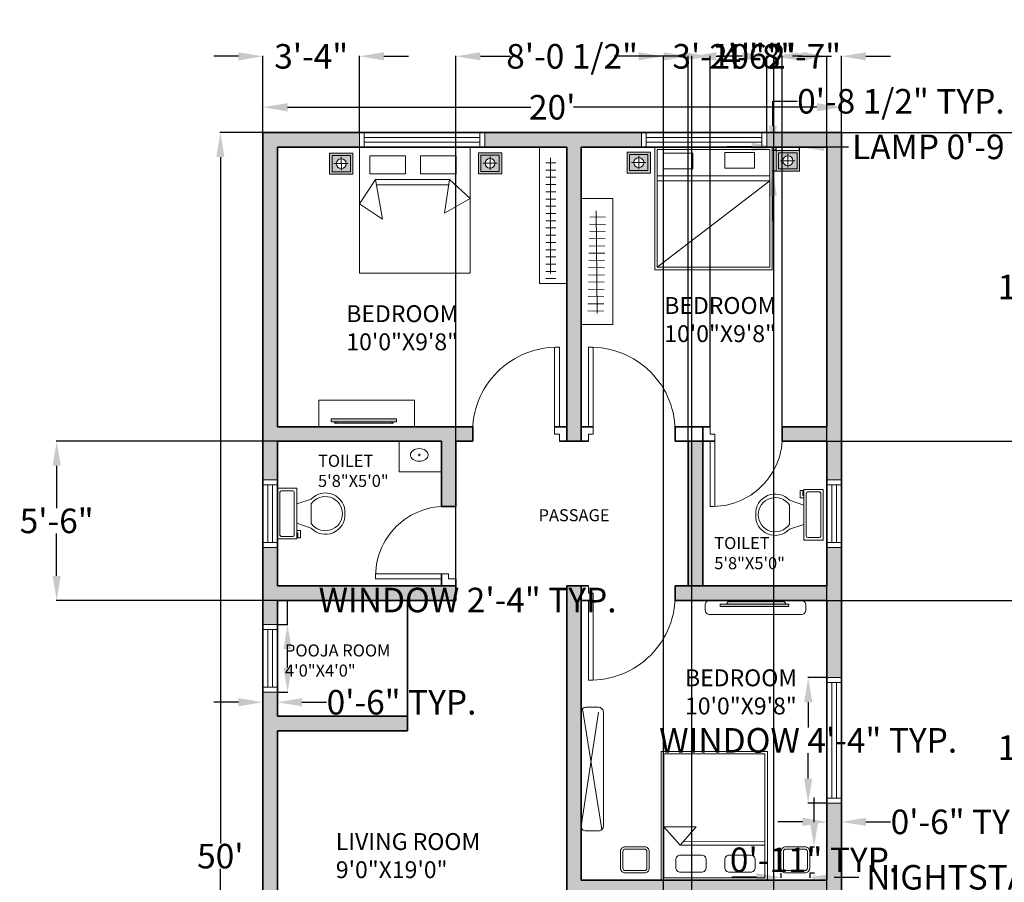
# Model space of a CAD drawing. Units: inches. Extents: x 1294 to 2470, y 659 to 1389.
# Tile 3 of 4: x 1306 to 1714, y 1031 to 1389. Entities that reach past the tile are written whole.
import ezdxf

# ---------------------------------------------------------------- set-up
doc = ezdxf.new("R2010")
doc.units = ezdxf.units.IN
doc.header["$MEASUREMENT"] = 0
for name, color, linetype, lineweight in [('A-ANNO-DIMS', 2, 'Continuous', 18), ('A-AREA-IDEN', 7, 'Continuous', 20), ('A-DOOR', 3, 'Continuous', 18), ('A-FLOR-CASE', 9, 'Continuous', 20), ('A-FLOR-FIXT', 9, 'Continuous', 18), ('A-FURN', 8, 'Continuous', 18), ('A-FURN-PATT', 9, 'Continuous', 13), ('A-GLAZ', 4, 'Continuous', 18), ('A-WALL', 7, 'Continuous', 35), ('A-WALL-PATT', 252, 'Continuous', 13)]:
    doc.layers.add(name, color=color, linetype=linetype, lineweight=lineweight)
doc.styles.get("Standard").update_dxf_attribs({"font": 'arial.ttf'})
doc.dimstyles.get("Standard").update_dxf_attribs({"dimtxt": 10.18, "dimasz": 10.18, "dimexe": 0.18, "dimexo": 0.0625, "dimgap": 0.09, "dimtad": 0, "dimtih": 1, "dimtoh": 1, "dimdec": 0, "dimzin": 0, "dimdsep": 46, "dimlunit": 3, "dimtxsty": 'Standard', "dimcen": 0.09, "dimadec": 0, "dimazin": 0, "dimtfac": 1, "dimtdec": 0, "dimtofl": 0, "dimtmove": 0, "dimatfit": 3, "dimfxl": 1, "dimtolj": 1, "dimtzin": 0, "dimarcsym": 0})

# ---------------------------------------------------------------- blocks, each defined once
blk = doc.blocks.new('*U2')
for p, q in [((9.5, -6), (9.5, -2)), ((-8, -8.5), (-8, -8)), ((-7, -8), (-7, -9.5)), ((-4, -8), (-6, -14)), ((4, -8), (6, -14)), ((-10, -8.5), (-8, -8.5)), ((-10, -9.5), (-10, -8.5)), ((-7, -9.5), (-10, -9.5)), ((4, -14), (-4, -14))]:
    blk.add_line(p, q)
blk.add_lwpolyline([(10.5, -8), (10.5, 0), (-10.5, 0), (-10.5, -8)], close=True)
for points in [[(-9.5, -2), (-9.5, -6)], [(8.5, -1), (-8.5, -1)], [(-8.5, -7), (8.5, -7)]]:
    blk.add_lwpolyline(points)
for centre, radius, start, end in [((-8.625, -1.875), 0.8839, 81.8699, 188.1301), ((8.625, -1.875), 0.8839, 351.8699, 98.1301), ((-8.625, -6.125), 0.8839, 171.869898, 278.1301), ((8.625, -6.125), 0.8839, 261.8699, 8.1301), ((-0.4772, -19.9188), 8.0953, 133.01722, 273.38), ((0.0374, -19.8731), 7.127, 124.50543, 269.7), ((-0.0373, -19.8731), 7.127, 270.3, 55.4946), ((0.4773, -19.9188), 8.0953, 266.62, 46.9828)]:
    blk.add_arc(centre, radius, start, end)
blk = doc.blocks.new('*D6')
at = {"layer": 'A-ANNO-DIMS', "color": 0, "lineweight": -2, "transparency": 16777216}
for p, q in [((1406.6, 1341.78), (1388.79, 1341.78)), ((1388.97, 1331.6), (1388.97, 1047.07)), ((1388.97, 751.96), (1388.97, 1036.5)), ((1406.6, 741.78), (1388.79, 741.78))]:
    blk.add_line(p, q, dxfattribs=at)
at = {"layer": 'A-ANNO-DIMS', "color": 0, "transparency": 16777216}
for points in [[(1387.28, 1331.6), (1390.67, 1331.6), (1388.97, 1341.78)], [(1387.28, 751.96), (1390.67, 751.96), (1388.97, 741.78)]]:
    blk.add_solid(points, dxfattribs=at)
at = {"layer": 'Defpoints', "color": 0, "transparency": 16777216}
for p in [(1406.66, 1341.78), (1388.97, 741.78), (1406.66, 741.78)]:
    blk.add_point(p, dxfattribs=at)
at = {"layer": 'A-ANNO-DIMS', "color": 0, "transparency": 16777216, "insert": (1388.97, 1041.78), "char_height": 10.18, "attachment_point": 5}
blk.add_mtext("\\A1;50'", dxfattribs=at)
blk = doc.blocks.new('*D7')
at = {"layer": 'A-ANNO-DIMS', "color": 0, "lineweight": -2, "transparency": 16777216}
for p, q in [((1406.66, 1341.85), (1406.66, 1352.45)), ((1416.84, 1352.27), (1517.85, 1352.27)), ((1636.48, 1352.27), (1535.48, 1352.27)), ((1646.66, 1341.85), (1646.66, 1352.45))]:
    blk.add_line(p, q, dxfattribs=at)
at = {"layer": 'A-ANNO-DIMS', "color": 0, "transparency": 16777216}
for points in [[(1416.84, 1353.97), (1416.84, 1350.57), (1406.66, 1352.27)], [(1636.48, 1353.97), (1636.48, 1350.57), (1646.66, 1352.27)]]:
    blk.add_solid(points, dxfattribs=at)
at = {"layer": 'Defpoints', "color": 0, "transparency": 16777216}
for p in [(1646.66, 1352.27), (1406.66, 1341.78), (1646.66, 1341.78)]:
    blk.add_point(p, dxfattribs=at)
at = {"layer": 'A-ANNO-DIMS', "color": 0, "transparency": 16777216, "insert": (1526.66, 1352.27), "char_height": 10.18, "attachment_point": 5}
blk.add_mtext("\\A1;20'", dxfattribs=at)
blk = doc.blocks.new('DOOR-SWING-36')
for p, q in [((34.01, 0), (34.01, 36)), ((36.01, 3), (36.01, 36)), ((34.01, 0), (36.01, 0))]:
    blk.add_line(p, q)
blk.add_arc((35.01, 1), 35.01, 88.3634, 181.6366)
blk = doc.blocks.new('WIN-48')
for p, q in [((0, 6), (0, 0)), ((2, 6), (2, 0)), ((50, 6), (50, 0)), ((52, 6), (52, 0)), ((50, 4), (2, 4)), ((50, 2), (2, 2))]:
    blk.add_line(p, q)
blk = doc.blocks.new('WIN-24')
for p, q in [((6, 28), (0, 28)), ((6, 26), (0, 26)), ((2, 26), (2, 2)), ((4, 26), (4, 2)), ((6, 2), (0, 2)), ((6, 0), (0, 0))]:
    blk.add_line(p, q)
blk = doc.blocks.new('NIGHTSTAND-LAMP')
h = blk.add_hatch(color=256)
h.dxf.hatch_style = 1
h.paths.add_polyline_path([(1, 7.67), (1, 1), (8.65, 1), (8.65, 7.67)], flags=0)
h.paths.add_polyline_path([(6.89, 4.34, -1), (2.76, 4.34, -1)], flags=0)
h.paths.add_polyline_path([(0, 8.67), (0, 0), (9.65, 0), (9.65, 8.67)])
h.paths.add_polyline_path([(8.65, 7.67), (8.65, 1), (1, 1), (1, 7.67)], flags=16)
h = blk.add_hatch(color=256)
h.dxf.hatch_style = 1
h.paths.add_polyline_path([(1, 7.67), (1, 1), (8.65, 1), (8.65, 7.67)])
h.paths.add_polyline_path([(6.89, 4.34, -1), (2.76, 4.34, -1)], flags=16)
for p, q in [((1.82, 4.38), (7.72, 4.39)), ((4.83, 7.2), (4.87, 1.61))]:
    blk.add_line(p, q)
for points in [[(9.65, 8.67), (0, 8.67), (0, 0), (9.65, 0)], [(8.65, 7.67), (1, 7.67), (1, 1), (8.65, 1)]]:
    blk.add_lwpolyline(points, close=True)
blk.add_circle((4.83, 4.34), 2.06)
blk = doc.blocks.new('NIGHTSTAND-RECT')
for points in [[(0, 8.9, -0.414214), (2, 10.9), (9.94, 10.9, -0.414214), (11.94, 8.9), (11.94, 2, -0.414214), (9.94, 0), (2, 0, -0.414214), (0, 2)], [(1, 8.9, -0.414214), (2, 9.9), (9.94, 9.9, -0.414214), (10.94, 8.9), (10.94, 2, -0.414214), (9.94, 1), (2, 1, -0.414214), (1, 2)]]:
    blk.add_lwpolyline(points, format="xyb", close=True)
blk = doc.blocks.new('*D18')
at = {"layer": 'A-ANNO-DIMS', "color": 0, "lineweight": -2, "transparency": 16777216}
for p, q in [((1640.6, 1115.78), (1632.68, 1115.78)), ((1632.86, 1105.6), (1632.86, 1095.14)), ((1632.86, 1073.96), (1632.86, 1084.43)), ((1640.6, 1063.78), (1632.68, 1063.78))]:
    blk.add_line(p, q, dxfattribs=at)
at = {"layer": 'A-ANNO-DIMS', "color": 0, "transparency": 16777216}
for points in [[(1631.17, 1105.6), (1634.56, 1105.6), (1632.86, 1115.78)], [(1631.17, 1073.96), (1634.56, 1073.96), (1632.86, 1063.78)]]:
    blk.add_solid(points, dxfattribs=at)
at = {"layer": 'Defpoints', "color": 0, "transparency": 16777216}
for p in [(1640.66, 1115.78), (1632.86, 1063.78), (1640.66, 1063.78)]:
    blk.add_point(p, dxfattribs=at)
at = {"layer": 'A-ANNO-DIMS', "color": 0, "transparency": 16777216, "insert": (1632.86, 1089.78), "char_height": 10.18, "attachment_point": 5}
blk.add_mtext('\\A1;WINDOW 4\'-4" TYP.', dxfattribs=at)
blk = doc.blocks.new('*D19')
at = {"layer": 'A-ANNO-DIMS', "color": 0, "lineweight": -2, "transparency": 16777216}
for p, q in [((1640.66, 1063.72), (1640.66, 1055.8)), ((1646.66, 1063.72), (1646.66, 1055.8)), ((1630.48, 1055.98), (1620.3, 1055.98)), ((1656.84, 1055.98), (1667.02, 1055.98))]:
    blk.add_line(p, q, dxfattribs=at)
at = {"layer": 'A-ANNO-DIMS', "color": 0, "transparency": 16777216}
for points in [[(1630.48, 1057.68), (1630.48, 1054.29), (1640.66, 1055.98)], [(1656.84, 1057.68), (1656.84, 1054.29), (1646.66, 1055.98)]]:
    blk.add_solid(points, dxfattribs=at)
at = {"layer": 'Defpoints', "color": 0, "transparency": 16777216}
for p in [(1640.66, 1063.78), (1646.66, 1063.78), (1646.66, 1055.98)]:
    blk.add_point(p, dxfattribs=at)
at = {"layer": 'A-ANNO-DIMS', "color": 0, "transparency": 16777216, "insert": (1698.14, 1055.98), "char_height": 10.18, "attachment_point": 5}
blk.add_mtext('\\A1;0\'-6" TYP.', dxfattribs=at)
blk = doc.blocks.new('*D20')
at = {"layer": 'A-ANNO-DIMS', "color": 0, "lineweight": -2, "transparency": 16777216}
for p, q in [((1416.86, 1137.78), (1416.86, 1147.96)), ((1416.86, 1147.96), (1427.04, 1147.96)), ((1412.72, 1137.78), (1417.04, 1137.78)), ((1416.86, 1119.96), (1416.86, 1127.6)), ((1412.72, 1109.78), (1417.04, 1109.78))]:
    blk.add_line(p, q, dxfattribs=at)
at = {"layer": 'A-ANNO-DIMS', "color": 0, "transparency": 16777216}
for points in [[(1415.17, 1127.6), (1418.56, 1127.6), (1416.86, 1137.78)], [(1415.17, 1119.96), (1418.56, 1119.96), (1416.86, 1109.78)]]:
    blk.add_solid(points, dxfattribs=at)
at = {"layer": 'Defpoints', "color": 0, "transparency": 16777216}
for p in [(1412.66, 1137.78), (1416.86, 1137.78), (1412.66, 1109.78)]:
    blk.add_point(p, dxfattribs=at)
at = {"layer": 'A-ANNO-DIMS', "color": 0, "transparency": 16777216, "insert": (1491.54, 1147.96), "char_height": 10.18, "attachment_point": 5}
blk.add_mtext('\\A1;WINDOW 2\'-4" TYP.', dxfattribs=at)
blk = doc.blocks.new('*D21')
at = {"layer": 'A-ANNO-DIMS', "color": 0, "lineweight": -2, "transparency": 16777216}
for p, q in [((1406.66, 1109.72), (1406.66, 1105.4)), ((1412.66, 1109.72), (1412.66, 1105.4)), ((1396.48, 1105.58), (1386.3, 1105.58)), ((1422.84, 1105.58), (1433.02, 1105.58))]:
    blk.add_line(p, q, dxfattribs=at)
at = {"layer": 'A-ANNO-DIMS', "color": 0, "transparency": 16777216}
for points in [[(1396.48, 1107.28), (1396.48, 1103.89), (1406.66, 1105.58)], [(1422.84, 1107.28), (1422.84, 1103.89), (1412.66, 1105.58)]]:
    blk.add_solid(points, dxfattribs=at)
at = {"layer": 'Defpoints', "color": 0, "transparency": 16777216}
for p in [(1406.66, 1109.78), (1412.66, 1109.78), (1412.66, 1105.58)]:
    blk.add_point(p, dxfattribs=at)
at = {"layer": 'A-ANNO-DIMS', "color": 0, "transparency": 16777216, "insert": (1464.14, 1105.58), "char_height": 10.18, "attachment_point": 5}
blk.add_mtext('\\A1;0\'-6" TYP.', dxfattribs=at)
blk = doc.blocks.new('*D24')
at = {"layer": 'A-ANNO-DIMS', "color": 0, "lineweight": -2, "transparency": 16777216}
for p, q in [((1609.43, 1335.84), (1599.25, 1335.84)), ((1619.61, 1334.46), (1619.61, 1336.02)), ((1629.26, 1334.46), (1629.26, 1336.02)), ((1639.44, 1335.84), (1649.62, 1335.84))]:
    blk.add_line(p, q, dxfattribs=at)
at = {"layer": 'A-ANNO-DIMS', "color": 0, "transparency": 16777216}
for points in [[(1609.43, 1337.54), (1609.43, 1334.14), (1619.61, 1335.84)], [(1639.44, 1337.54), (1639.44, 1334.14), (1629.26, 1335.84)]]:
    blk.add_solid(points, dxfattribs=at)
at = {"layer": 'Defpoints', "color": 0, "transparency": 16777216}
for p in [(1629.26, 1335.84), (1619.61, 1334.39), (1629.26, 1334.39)]:
    blk.add_point(p, dxfattribs=at)
at = {"layer": 'A-ANNO-DIMS', "color": 0, "transparency": 16777216, "insert": (1713.71, 1335.84), "char_height": 10.18, "attachment_point": 5}
blk.add_mtext('\\A1;LAMP 0\'-9 1/2" TYP.', dxfattribs=at)
blk = doc.blocks.new('*D25')
at = {"layer": 'A-ANNO-DIMS', "color": 0, "lineweight": -2, "transparency": 16777216}
for p, q in [((1618.16, 1344.57), (1618.16, 1354.75)), ((1618.16, 1354.75), (1628.34, 1354.75)), ((1619.55, 1334.39), (1617.98, 1334.39)), ((1619.55, 1325.72), (1617.98, 1325.72)), ((1618.16, 1315.54), (1618.16, 1305.36))]:
    blk.add_line(p, q, dxfattribs=at)
at = {"layer": 'A-ANNO-DIMS', "color": 0, "transparency": 16777216}
for points in [[(1616.47, 1344.57), (1619.86, 1344.57), (1618.16, 1334.39)], [(1616.47, 1315.54), (1619.86, 1315.54), (1618.16, 1325.72)]]:
    blk.add_solid(points, dxfattribs=at)
at = {"layer": 'Defpoints', "color": 0, "transparency": 16777216}
for p in [(1618.16, 1334.39), (1619.61, 1334.39), (1619.61, 1325.72)]:
    blk.add_point(p, dxfattribs=at)
at = {"layer": 'A-ANNO-DIMS', "color": 0, "transparency": 16777216, "insert": (1671.32, 1354.75), "char_height": 10.18, "attachment_point": 5}
blk.add_mtext('\\A1;0\'-8 1/2" TYP.', dxfattribs=at)
blk = doc.blocks.new('*D26')
at = {"layer": 'A-ANNO-DIMS', "color": 0, "lineweight": -2, "transparency": 16777216}
for p, q in [((1621.57, 1034.72), (1621.57, 1032.82)), ((1633.51, 1034.72), (1633.51, 1032.82)), ((1611.39, 1033), (1601.21, 1033)), ((1643.69, 1033), (1653.87, 1033))]:
    blk.add_line(p, q, dxfattribs=at)
at = {"layer": 'A-ANNO-DIMS', "color": 0, "transparency": 16777216}
for points in [[(1611.39, 1034.69), (1611.39, 1031.3), (1621.57, 1033)], [(1643.69, 1034.69), (1643.69, 1031.3), (1633.51, 1033)]]:
    blk.add_solid(points, dxfattribs=at)
at = {"layer": 'Defpoints', "color": 0, "transparency": 16777216}
for p in [(1621.57, 1034.79), (1633.51, 1034.79), (1633.51, 1033)]:
    blk.add_point(p, dxfattribs=at)
at = {"layer": 'A-ANNO-DIMS', "color": 0, "transparency": 16777216, "insert": (1732.93, 1033), "char_height": 10.18, "attachment_point": 5}
blk.add_mtext('\\A1;NIGHTSTAND 1\'-0" TYP.', dxfattribs=at)
blk = doc.blocks.new('*D27')
at = {"layer": 'A-ANNO-DIMS', "color": 0, "lineweight": -2, "transparency": 16777216}
for p, q in [((1635.3, 1055.87), (1635.3, 1066.05)), ((1633.57, 1045.69), (1635.48, 1045.69)), ((1633.57, 1034.79), (1635.48, 1034.79)), ((1635.3, 1024.61), (1635.3, 1014.43))]:
    blk.add_line(p, q, dxfattribs=at)
at = {"layer": 'A-ANNO-DIMS', "color": 0, "transparency": 16777216}
for points in [[(1633.6, 1055.87), (1637, 1055.87), (1635.3, 1045.69)], [(1633.6, 1024.61), (1637, 1024.61), (1635.3, 1034.79)]]:
    blk.add_solid(points, dxfattribs=at)
at = {"layer": 'Defpoints', "color": 0, "transparency": 16777216}
for p in [(1633.51, 1045.69), (1635.3, 1045.69), (1633.51, 1034.79)]:
    blk.add_point(p, dxfattribs=at)
at = {"layer": 'A-ANNO-DIMS', "color": 0, "transparency": 16777216, "insert": (1635.3, 1040.24), "char_height": 10.18, "attachment_point": 5}
blk.add_mtext('\\A1;0\'-11" TYP.', dxfattribs=at)
blk = doc.blocks.new('*D39')
at = {"layer": 'A-ANNO-DIMS', "color": 0, "lineweight": -2, "transparency": 16777216}
for p, q in [((1640.72, 1147.78), (1730.86, 1147.78)), ((1730.68, 1137.6), (1730.68, 1092.07)), ((1730.68, 1035.96), (1730.68, 1081.5)), ((1640.72, 1025.78), (1730.86, 1025.78))]:
    blk.add_line(p, q, dxfattribs=at)
at = {"layer": 'A-ANNO-DIMS', "color": 0, "transparency": 16777216}
for points in [[(1728.99, 1137.6), (1732.38, 1137.6), (1730.68, 1147.78)], [(1728.99, 1035.96), (1732.38, 1035.96), (1730.68, 1025.78)]]:
    blk.add_solid(points, dxfattribs=at)
at = {"layer": 'Defpoints', "color": 0, "transparency": 16777216}
for p in [(1640.66, 1147.78), (1730.68, 1147.78), (1640.66, 1025.78)]:
    blk.add_point(p, dxfattribs=at)
at = {"layer": 'A-ANNO-DIMS', "color": 0, "transparency": 16777216, "insert": (1730.68, 1086.78), "char_height": 10.18, "attachment_point": 5}
blk.add_mtext('\\A1;10\'-2"', dxfattribs=at)
blk = doc.blocks.new('*D40')
at = {"layer": 'A-ANNO-DIMS', "color": 0, "lineweight": -2, "transparency": 16777216}
for p, q in [((1412.6, 1213.78), (1320.88, 1213.78)), ((1321.06, 1203.6), (1321.06, 1186.07)), ((1321.06, 1157.96), (1321.06, 1175.5)), ((1412.6, 1147.78), (1320.88, 1147.78))]:
    blk.add_line(p, q, dxfattribs=at)
at = {"layer": 'A-ANNO-DIMS', "color": 0, "transparency": 16777216}
for points in [[(1319.37, 1203.6), (1322.76, 1203.6), (1321.06, 1213.78)], [(1319.37, 1157.96), (1322.76, 1157.96), (1321.06, 1147.78)]]:
    blk.add_solid(points, dxfattribs=at)
at = {"layer": 'Defpoints', "color": 0, "transparency": 16777216}
for p in [(1321.06, 1213.78), (1412.66, 1213.78), (1412.66, 1147.78)]:
    blk.add_point(p, dxfattribs=at)
at = {"layer": 'A-ANNO-DIMS', "color": 0, "transparency": 16777216, "insert": (1321.06, 1180.78), "char_height": 10.18, "attachment_point": 5}
blk.add_mtext('\\A1;5\'-6"', dxfattribs=at)
blk = doc.blocks.new('*D41')
at = {"layer": 'A-ANNO-DIMS', "color": 0, "lineweight": -2, "transparency": 16777216}
for p, q in [((1646.72, 1341.78), (1730.86, 1341.78)), ((1730.68, 1331.6), (1730.68, 1283.07)), ((1730.68, 1223.96), (1730.68, 1272.5)), ((1640.72, 1213.78), (1730.86, 1213.78))]:
    blk.add_line(p, q, dxfattribs=at)
at = {"layer": 'A-ANNO-DIMS', "color": 0, "transparency": 16777216}
for points in [[(1728.99, 1331.6), (1732.38, 1331.6), (1730.68, 1341.78)], [(1728.99, 1223.96), (1732.38, 1223.96), (1730.68, 1213.78)]]:
    blk.add_solid(points, dxfattribs=at)
at = {"layer": 'Defpoints', "color": 0, "transparency": 16777216}
for p in [(1646.66, 1341.78), (1730.68, 1341.78), (1640.66, 1213.78)]:
    blk.add_point(p, dxfattribs=at)
at = {"layer": 'A-ANNO-DIMS', "color": 0, "transparency": 16777216, "insert": (1730.68, 1277.78), "char_height": 10.18, "attachment_point": 5}
blk.add_mtext('\\A1;10\'-8"', dxfattribs=at)
blk = doc.blocks.new('*D42')
at = {"layer": 'A-ANNO-DIMS', "color": 0, "lineweight": -2, "transparency": 16777216}
for p, q in [((1396.48, 1373.38), (1386.3, 1373.38)), ((1406.66, 1341.85), (1406.66, 1373.56)), ((1446.66, 1341.85), (1446.66, 1373.56)), ((1456.84, 1373.38), (1467.02, 1373.38))]:
    blk.add_line(p, q, dxfattribs=at)
at = {"layer": 'A-ANNO-DIMS', "color": 0, "transparency": 16777216}
for points in [[(1396.48, 1375.08), (1396.48, 1371.69), (1406.66, 1373.38)], [(1456.84, 1375.08), (1456.84, 1371.69), (1446.66, 1373.38)]]:
    blk.add_solid(points, dxfattribs=at)
at = {"layer": 'Defpoints', "color": 0, "transparency": 16777216}
for p in [(1446.66, 1373.38), (1406.66, 1341.78), (1446.66, 1341.78)]:
    blk.add_point(p, dxfattribs=at)
at = {"layer": 'A-ANNO-DIMS', "color": 0, "transparency": 16777216, "insert": (1426.66, 1373.38), "char_height": 10.18, "attachment_point": 5}
blk.add_mtext('\\A1;3\'-4"', dxfattribs=at)
blk = doc.blocks.new('*D43')
at = {"layer": 'A-ANNO-DIMS', "color": 0, "lineweight": -2, "transparency": 16777216}
for p, q in [((1605.48, 1373.38), (1595.3, 1373.38)), ((1615.66, 1341.85), (1615.66, 1373.56)), ((1646.66, 1341.85), (1646.66, 1373.56)), ((1656.84, 1373.38), (1667.02, 1373.38))]:
    blk.add_line(p, q, dxfattribs=at)
at = {"layer": 'A-ANNO-DIMS', "color": 0, "transparency": 16777216}
for points in [[(1605.48, 1375.08), (1605.48, 1371.69), (1615.66, 1373.38)], [(1656.84, 1375.08), (1656.84, 1371.69), (1646.66, 1373.38)]]:
    blk.add_solid(points, dxfattribs=at)
at = {"layer": 'Defpoints', "color": 0, "transparency": 16777216}
for p in [(1646.66, 1373.38), (1615.66, 1341.78), (1646.66, 1341.78)]:
    blk.add_point(p, dxfattribs=at)
at = {"layer": 'A-ANNO-DIMS', "color": 0, "transparency": 16777216, "insert": (1631.16, 1373.38), "char_height": 10.18, "attachment_point": 5}
blk.add_mtext('\\A1;2\'-7"', dxfattribs=at)
blk = doc.blocks.new('*D44')
at = {"layer": 'A-ANNO-DIMS', "color": 0, "lineweight": -2, "transparency": 16777216}
for p, q in [((1486.66, 1153.85), (1486.66, 1373.56)), ((1496.84, 1373.38), (1509.41, 1373.38)), ((1572.95, 1373.38), (1560.38, 1373.38)), ((1583.13, 1153.85), (1583.13, 1373.56))]:
    blk.add_line(p, q, dxfattribs=at)
at = {"layer": 'A-ANNO-DIMS', "color": 0, "transparency": 16777216}
for points in [[(1496.84, 1375.08), (1496.84, 1371.69), (1486.66, 1373.38)], [(1572.95, 1375.08), (1572.95, 1371.69), (1583.13, 1373.38)]]:
    blk.add_solid(points, dxfattribs=at)
at = {"layer": 'Defpoints', "color": 0, "transparency": 16777216}
for p in [(1583.13, 1373.38), (1486.66, 1153.78), (1583.13, 1153.78)]:
    blk.add_point(p, dxfattribs=at)
at = {"layer": 'A-ANNO-DIMS', "color": 0, "transparency": 16777216, "insert": (1534.9, 1373.38), "char_height": 10.18, "attachment_point": 5}
blk.add_mtext('\\A1;8\'-0 1/2"', dxfattribs=at)
blk = doc.blocks.new('*D45')
at = {"layer": 'A-ANNO-DIMS', "color": 0, "lineweight": -2, "transparency": 16777216}
for p, q in [((1581.95, 1373.38), (1571.77, 1373.38)), ((1592.13, 1219.85), (1592.13, 1373.56)), ((1622.13, 1219.85), (1622.13, 1373.56)), ((1632.31, 1373.38), (1642.49, 1373.38))]:
    blk.add_line(p, q, dxfattribs=at)
at = {"layer": 'A-ANNO-DIMS', "color": 0, "transparency": 16777216}
for points in [[(1581.95, 1375.08), (1581.95, 1371.69), (1592.13, 1373.38)], [(1632.31, 1375.08), (1632.31, 1371.69), (1622.13, 1373.38)]]:
    blk.add_solid(points, dxfattribs=at)
at = {"layer": 'Defpoints', "color": 0, "transparency": 16777216}
for p in [(1622.13, 1373.38), (1592.13, 1219.78), (1622.13, 1219.78)]:
    blk.add_point(p, dxfattribs=at)
at = {"layer": 'A-ANNO-DIMS', "color": 0, "transparency": 16777216, "insert": (1607.13, 1373.38), "char_height": 10.18, "attachment_point": 5}
blk.add_mtext('\\A1;2\'-6"', dxfattribs=at)
blk = doc.blocks.new('*D50')
at = {"layer": 'A-ANNO-DIMS', "color": 0, "lineweight": -2, "transparency": 16777216}
for p, q in [((1562.59, 1373.38), (1552.41, 1373.38)), ((1572.77, 1001.97), (1572.77, 1373.56)), ((1618.65, 1001.97), (1618.65, 1373.56)), ((1628.83, 1373.38), (1639.01, 1373.38))]:
    blk.add_line(p, q, dxfattribs=at)
at = {"layer": 'A-ANNO-DIMS', "color": 0, "transparency": 16777216}
for points in [[(1562.59, 1375.08), (1562.59, 1371.69), (1572.77, 1373.38)], [(1628.83, 1375.08), (1628.83, 1371.69), (1618.65, 1373.38)]]:
    blk.add_solid(points, dxfattribs=at)
at = {"layer": 'Defpoints', "color": 0, "transparency": 16777216}
for p in [(1618.65, 1373.38), (1572.77, 1001.91), (1618.65, 1001.91)]:
    blk.add_point(p, dxfattribs=at)
at = {"layer": 'A-ANNO-DIMS', "color": 0, "transparency": 16777216, "insert": (1595.71, 1373.38), "char_height": 10.18, "attachment_point": 5}
blk.add_mtext('\\A1;3\'-10"', dxfattribs=at)
blk = doc.blocks.new('*D53')
at = {"layer": 'A-ANNO-DIMS', "color": 0, "lineweight": -2, "transparency": 16777216}
for p, q in [((1584.52, 951.85), (1584.52, 1373.56)), ((1594.7, 1373.38), (1598.77, 1373.38)), ((1630.48, 1373.38), (1626.42, 1373.38)), ((1640.66, 951.85), (1640.66, 1373.56))]:
    blk.add_line(p, q, dxfattribs=at)
at = {"layer": 'A-ANNO-DIMS', "color": 0, "transparency": 16777216}
for points in [[(1594.7, 1375.08), (1594.7, 1371.69), (1584.52, 1373.38)], [(1630.48, 1375.08), (1630.48, 1371.69), (1640.66, 1373.38)]]:
    blk.add_solid(points, dxfattribs=at)
at = {"layer": 'Defpoints', "color": 0, "transparency": 16777216}
for p in [(1640.66, 1373.38), (1584.52, 951.78), (1640.66, 951.78)]:
    blk.add_point(p, dxfattribs=at)
at = {"layer": 'A-ANNO-DIMS', "color": 0, "transparency": 16777216, "insert": (1612.59, 1373.38), "char_height": 10.18, "attachment_point": 5}
blk.add_mtext('\\A1;4\'-8"', dxfattribs=at)

msp = doc.modelspace()

# ---------------------------------------------------------------- hatches: boundary and pattern name
at = {"layer": 'A-FURN-PATT'}
h = msp.add_hatch(color=256, dxfattribs=at)
h.dxf.hatch_style = 1
h.paths.add_polyline_path([(1504.69, 1332.37), (1497.04, 1332.37), (1497.04, 1325.69), (1504.69, 1325.69)], flags=0)
h.paths.add_polyline_path([(1502.93, 1329.03, -1), (1498.8, 1329.03, -1)], flags=0)
h.paths.add_polyline_path([(1505.69, 1333.37), (1496.04, 1333.37), (1496.04, 1324.69), (1505.69, 1324.69)])
h.paths.add_polyline_path([(1504.69, 1332.37), (1504.69, 1325.69), (1497.04, 1325.69), (1497.04, 1332.37)], flags=16)
h = msp.add_hatch(color=256, dxfattribs=at)
h.dxf.hatch_style = 1
h.paths.add_polyline_path([(1504.69, 1332.37), (1497.04, 1332.37), (1497.04, 1325.69), (1504.69, 1325.69)])
h.paths.add_polyline_path([(1502.93, 1329.03, -1), (1498.8, 1329.03, -1)], flags=16)
h = msp.add_hatch(color=256, dxfattribs=at)
h.dxf.hatch_style = 1
h.paths.add_polyline_path([(1462.1, 1223.05), (1434.93, 1223.05), (1434.93, 1221.9), (1462.1, 1221.9)])
h.paths.add_polyline_path([(1459.75, 1221.9), (1437.6, 1221.9), (1436.14, 1221.32), (1460.75, 1221.32)])
h = msp.add_hatch(color=256, dxfattribs=at)
h.dxf.hatch_style = 1
h.paths.add_polyline_path([(1599.68, 1147.35), (1599, 1146.28), (1623.79, 1146.28), (1622.94, 1147.29)])
h.paths.add_polyline_path([(1596.38, 1146.28), (1596.38, 1145.27), (1624.84, 1145.27), (1624.84, 1146.28)])
at = {"layer": 'A-WALL-PATT'}
h = msp.add_hatch(color=256, dxfattribs=at)
h.dxf.hatch_style = 1
h.paths.add_polyline_path([(1412.66, 1335.78), (1446.66, 1335.78), (1446.66, 1341.78), (1406.66, 1341.78), (1406.66, 1197.78), (1412.66, 1197.78), (1412.66, 1213.78), (1480.66, 1213.78), (1480.66, 1186.78), (1481.11, 1186.78, -0.021978), (1483.66, 1186.78), (1486.66, 1186.78), (1486.66, 1213.78), (1493.66, 1213.78), (1493.66, 1216.78, -0.014283), (1493.66, 1218.78), (1493.66, 1219.78), (1412.66, 1219.78)])
h.paths.add_polyline_path([(1563.66, 1341.78), (1498.66, 1341.78), (1498.66, 1335.78), (1532.66, 1335.78), (1532.66, 1219.78), (1532.66, 1213.78), (1538.66, 1213.78), (1538.66, 1219.78), (1538.66, 1335.78), (1563.66, 1335.78)])
h.paths.add_polyline_path([(1646.66, 1341.78), (1615.66, 1341.78), (1615.66, 1335.78), (1640.66, 1335.78), (1640.66, 1219.78), (1622.13, 1219.78), (1622.13, 1216.78, -0.017236), (1622.13, 1214.78), (1622.13, 1213.78), (1640.66, 1213.78), (1640.66, 1197.78), (1646.66, 1197.78)])
h.paths.add_polyline_path([(1646.66, 1169.78), (1640.66, 1169.78), (1640.66, 1153.78), (1577.66, 1153.78), (1577.66, 1150.78, -0.014283), (1577.66, 1148.78), (1577.66, 1147.78), (1640.66, 1147.78), (1640.66, 1115.78), (1646.66, 1115.78)])
h.paths.add_polyline_path([(1589.13, 1213.78), (1583.13, 1213.78), (1583.13, 1153.78), (1589.13, 1153.78)])
h.paths.add_polyline_path([(1538.66, 1147.78), (1538.66, 1153.78), (1532.66, 1153.78), (1532.66, 1025.78), (1538.66, 1025.78), (1640.66, 1025.78), (1640.66, 971.78), (1646.66, 971.78), (1646.66, 1063.78), (1640.66, 1063.78), (1640.66, 1031.78), (1538.66, 1031.78)])
h.paths.add_polyline_path([(1486.66, 1153.78), (1480.66, 1153.78), (1412.66, 1153.78), (1412.66, 1169.78), (1406.66, 1169.78), (1406.66, 1137.78), (1412.66, 1137.78), (1412.66, 1147.78), (1460.66, 1147.78), (1466.66, 1147.78), (1486.66, 1147.78)])
h.paths.add_polyline_path([(1466.66, 1099.78), (1460.66, 1099.78), (1412.66, 1099.78), (1412.66, 1109.78), (1406.66, 1109.78), (1406.66, 1005.78), (1412.66, 1005.78), (1412.66, 1093.78), (1466.66, 1093.78)])
h.paths.add_polyline_path([(1412.66, 953.78), (1406.66, 953.78), (1406.66, 741.78), (1433.66, 741.78), (1433.66, 747.78), (1412.66, 747.78), (1412.66, 859.78), (1493.66, 859.78), (1493.66, 862.78, -0.014283), (1493.66, 864.78), (1493.66, 865.78), (1412.66, 865.78)])
h.paths.add_polyline_path([(1538.66, 988.41), (1532.66, 988.41), (1532.66, 865.78), (1532.66, 859.78), (1538.66, 859.78), (1640.66, 859.78), (1640.66, 747.78), (1538.66, 747.78), (1532.66, 747.78), (1511.66, 747.78), (1511.66, 741.78), (1646.66, 741.78), (1646.66, 919.78), (1640.66, 919.78), (1640.66, 865.78), (1538.66, 865.78)])

# ---------------------------------------------------------------- linework, layer by layer
at = {"layer": 'A-DOOR'}
for p, q in [((1592.13, 1216.78), (1592.13, 1219.78)), ((1529.66, 1216.78), (1529.66, 1213.78)), ((1541.66, 1216.78), (1541.66, 1213.78)), ((1594.13, 1216.78), (1592.13, 1216.78)), ((1592.13, 1213.78), (1592.13, 1186.78)), ((1594.13, 1216.78), (1594.13, 1186.78)), ((1483.66, 1158.78), (1453.38, 1158.78)), ((1480.66, 1156.78), (1453.38, 1156.78)), ((1453.38, 1156.78), (1453.38, 1156.78)), ((1483.66, 1158.78), (1483.66, 1156.78)), ((1483.66, 1156.78), (1486.66, 1156.78)), ((1541.66, 1150.78), (1541.66, 1153.78))]:
    msp.add_line(p, q, dxfattribs=at)
for centre, radius, start, end in [((1593.13, 1215.78), 29.02, 268.0251, 1.9749), ((1482.39, 1157.78), 29.03, 87.4819, 181.9742)]:
    msp.add_arc(centre, radius, start, end, dxfattribs=at)
at = {"layer": 'A-FLOR-CASE'}
for p, q in [((1521.4, 1335.78), (1521.4, 1279.14)), ((1524.07, 1329.22), (1528.1, 1329.22)), ((1526.01, 1331.26), (1526.01, 1283.34)), ((1524.07, 1326.22), (1528.1, 1326.22)), ((1524.07, 1323.22), (1528.1, 1323.22)), ((1524.07, 1320.22), (1528.1, 1320.22)), ((1524.07, 1317.22), (1528.1, 1317.22)), ((1524.07, 1314.22), (1528.1, 1314.22)), ((1524.07, 1311.22), (1528.1, 1311.22)), ((1524.07, 1308.22), (1528.1, 1308.22)), ((1544.96, 1309.37), (1545.3, 1266.93)), ((1524.07, 1305.22), (1528.1, 1305.22)), ((1542.13, 1303.83), (1548.72, 1303.69)), ((1542.2, 1306.83), (1548.78, 1306.69)), ((1524.07, 1302.22), (1528.1, 1302.22)), ((1524.07, 1299.22), (1528.1, 1299.22)), ((1542.07, 1300.83), (1548.66, 1300.69)), ((1524.07, 1296.22), (1528.1, 1296.22)), ((1542.01, 1297.83), (1548.6, 1297.69)), ((1524.07, 1293.22), (1528.1, 1293.22)), ((1541.89, 1291.83), (1548.48, 1291.7)), ((1541.95, 1294.83), (1548.54, 1294.69)), ((1524.07, 1290.22), (1528.1, 1290.22)), ((1524.07, 1287.22), (1528.1, 1287.22)), ((1541.83, 1288.83), (1548.42, 1288.7)), ((1524.07, 1284.22), (1528.1, 1284.22)), ((1541.71, 1282.83), (1548.29, 1282.7)), ((1541.77, 1285.83), (1548.36, 1285.7)), ((1521.4, 1279.14), (1532.66, 1279.14)), ((1524.07, 1281.22), (1528.1, 1281.22)), ((1541.65, 1279.83), (1548.23, 1279.7)), ((1541.58, 1276.83), (1548.17, 1276.7)), ((1541.46, 1270.83), (1548.05, 1270.7)), ((1541.52, 1273.83), (1548.11, 1273.7)), ((1541.4, 1267.83), (1547.99, 1267.7))]:
    msp.add_line(p, q, dxfattribs=at)
msp.add_lwpolyline([(1538.66, 1314.46), (1551.76, 1314.46), (1551.76, 1262.18), (1538.66, 1262.18)], close=True, dxfattribs=at)
at = {"layer": 'A-FLOR-FIXT'}
msp.add_lwpolyline([(1480.66, 1213.78), (1480.66, 1213.78), (1463.1, 1213.78), (1463.1, 1213.78), (1463.1, 1201.16), (1463.1, 1201.16), (1480.66, 1201.16), (1480.66, 1201.16)], close=True, dxfattribs=at)
msp.add_circle((1471.52, 1208.13), 0.361, dxfattribs=at)
msp.add_ellipse((1471.52, 1208.13), major_axis=(-3.67, 0), ratio=0.71736, dxfattribs=at)
at = {"layer": 'A-FURN'}
for p, q in [((1500.87, 1331.89), (1500.91, 1326.3)), ((1497.86, 1329.07), (1503.76, 1329.08)), ((1570.2, 1323.81), (1616.94, 1323.81)), ((1446.66, 1323.19), (1446.66, 1323.19)), ((1453.4, 1322.34), (1446.66, 1312.28)), ((1453.4, 1322.34), (1484.03, 1322.34)), ((1456.3, 1305.82), (1453.4, 1322.34)), ((1453.79, 1320.14), (1483.71, 1320.08)), ((1482.03, 1308.3), (1484.03, 1322.34)), ((1484.03, 1322.34), (1492.63, 1314.42)), ((1570.2, 1321.81), (1616.94, 1321.81)), ((1570.2, 1285.9), (1616.94, 1321.81)), ((1446.66, 1312.28), (1456.3, 1305.82)), ((1492.63, 1314.42), (1482.03, 1308.3)), ((1437.6, 1221.9), (1436.14, 1221.32)), ((1460.75, 1221.32), (1459.75, 1221.9)), ((1436.14, 1221.32), (1460.75, 1221.32)), ((1599, 1146.28), (1599.68, 1147.35)), ((1599.68, 1147.35), (1622.94, 1147.29)), ((1622.94, 1147.29), (1623.79, 1146.28)), ((1545.89, 1101.49), (1538.66, 1054.22)), ((1539.25, 1102.9), (1547.3, 1052.8)), ((1579.69, 1046.28), (1572.91, 1053.98)), ((1572.91, 1053.98), (1586.42, 1053.98)), ((1586.42, 1053.98), (1579.69, 1046.28)), ((1614.93, 1046.28), (1579.69, 1046.28)), ((1614.93, 1047.84), (1580.95, 1047.72)), ((1614.93, 1046.28), (1614.93, 1046.28))]:
    msp.add_line(p, q, dxfattribs=at)
for points in [[(1446.66, 1335.78), (1492.63, 1335.78), (1492.63, 1283.41), (1446.66, 1283.41)], [(1450.96, 1332.18), (1465.82, 1332.18), (1465.82, 1324.7), (1450.96, 1324.7)], [(1471.95, 1332.18), (1486.8, 1332.18), (1486.8, 1324.7), (1471.95, 1324.7)], [(1505.69, 1333.37), (1496.04, 1333.37), (1496.04, 1324.69), (1505.69, 1324.69)], [(1504.69, 1332.37), (1497.04, 1332.37), (1497.04, 1325.69), (1504.69, 1325.69)], [(1617.94, 1335.78), (1569.2, 1335.78), (1569.2, 1284.9), (1617.94, 1284.9)], [(1616.94, 1334.78), (1570.2, 1334.78), (1570.2, 1285.9), (1616.94, 1285.9)], [(1572.77, 1333.23), (1585.06, 1333.23), (1585.06, 1326.8), (1572.77, 1326.8)], [(1598.24, 1333.46), (1610.53, 1333.46), (1610.53, 1327.02), (1598.24, 1327.02)], [(1469.46, 1219.78), (1429.82, 1219.78), (1429.82, 1230.79), (1469.46, 1230.79)], [(1434.93, 1223.05), (1462.1, 1223.05), (1462.1, 1221.9), (1434.93, 1221.9)], [(1596.38, 1146.28), (1596.38, 1146.28), (1624.84, 1146.28), (1624.84, 1146.28), (1624.84, 1145.27), (1624.84, 1145.27), (1596.38, 1145.27), (1596.38, 1145.27)], [(1571.91, 1031.78), (1615.93, 1031.78), (1615.93, 1085.14), (1571.91, 1085.14)], [(1572.91, 1032.78), (1614.93, 1032.78), (1614.93, 1084.14), (1572.91, 1084.14)]]:
    msp.add_lwpolyline(points, close=True, dxfattribs=at)
for points in [[(1590.06, 1145.78, -0.414214), (1592.06, 1147.78), (1629.94, 1147.78, -0.414214), (1631.94, 1145.78), (1631.94, 1143.94, -0.414214), (1629.94, 1141.94), (1592.06, 1141.94, -0.414214), (1590.06, 1143.94)], [(1538.66, 1101.49, -0.414214), (1540.66, 1103.49), (1545.89, 1103.49, -0.414214), (1547.89, 1101.49), (1547.89, 1054.22, -0.414214), (1545.89, 1052.22), (1540.66, 1052.22, -0.414214), (1538.66, 1054.22)], [(1577.89, 1040.17, -0.414214), (1579.89, 1042.17), (1588.54, 1042.17, -0.414214), (1590.54, 1040.17), (1590.54, 1037.12, -0.414214), (1588.54, 1035.12), (1579.89, 1035.12, -0.414214), (1577.89, 1037.12)], [(1598.24, 1040.17, -0.414214), (1600.24, 1042.17), (1608.89, 1042.17, -0.414214), (1610.89, 1040.17), (1610.89, 1037.12, -0.414214), (1608.89, 1035.12), (1600.24, 1035.12, -0.414214), (1598.24, 1037.12)]]:
    msp.add_lwpolyline(points, format="xyb", close=True, dxfattribs=at)
msp.add_circle((1500.87, 1329.03), 2.06, dxfattribs=at)
at = {"layer": 'A-WALL'}
for p, q in [((1406.66, 741.78), (1406.66, 1341.78)), ((1406.66, 1341.78), (1646.66, 1341.78)), ((1646.66, 1341.78), (1646.66, 741.78)), ((1412.66, 1335.78), (1532.66, 1335.78)), ((1412.66, 1219.78), (1412.66, 1335.78)), ((1532.66, 1219.78), (1532.66, 1335.78)), ((1538.66, 1219.78), (1538.66, 1335.78)), ((1538.66, 1335.78), (1640.66, 1335.78)), ((1640.66, 1335.78), (1640.66, 1219.78)), ((1412.66, 1219.78), (1493.7, 1219.78)), ((1493.66, 1219.78), (1493.66, 1213.78)), ((1527.66, 1219.78), (1532.66, 1219.78)), ((1532.66, 1219.78), (1532.66, 1213.78)), ((1538.66, 1219.78), (1543.66, 1219.78)), ((1538.66, 1219.78), (1538.66, 1213.78)), ((1577.62, 1219.78), (1592.13, 1219.78)), ((1577.66, 1219.78), (1577.66, 1213.78)), ((1589.13, 1213.78), (1589.13, 1219.78)), ((1622.13, 1213.78), (1622.13, 1219.78)), ((1622.13, 1219.78), (1640.66, 1219.78)), ((1412.66, 1213.78), (1480.66, 1213.78)), ((1412.66, 1153.78), (1412.66, 1213.78)), ((1480.66, 1186.76), (1480.66, 1213.78)), ((1486.66, 1213.78), (1493.66, 1213.78)), ((1486.66, 1186.78), (1486.66, 1213.78)), ((1529.66, 1213.78), (1541.66, 1213.78)), ((1577.66, 1213.78), (1594.13, 1213.78)), ((1583.13, 1213.78), (1583.13, 1153.78)), ((1589.13, 1213.78), (1589.13, 1153.78)), ((1622.08, 1213.78), (1640.66, 1213.78)), ((1640.66, 1213.78), (1640.66, 1153.78)), ((1480.66, 1186.78), (1486.66, 1186.78)), ((1480.66, 1153.78), (1480.66, 1158.78)), ((1486.66, 1147.78), (1486.66, 1156.78)), ((1412.66, 1153.78), (1480.66, 1153.78)), ((1412.66, 1153.78), (1480.66, 1153.78)), ((1480.66, 1153.78), (1486.66, 1153.78)), ((1532.66, 1153.78), (1541.66, 1153.78)), ((1532.66, 1025.78), (1532.66, 1153.78)), ((1538.66, 1147.78), (1538.66, 1153.78)), ((1577.66, 1153.78), (1640.66, 1153.78)), ((1577.66, 1147.78), (1577.66, 1153.78)), ((1412.66, 1147.78), (1460.66, 1147.78)), ((1412.66, 1147.78), (1460.66, 1147.78)), ((1412.66, 1099.78), (1412.66, 1147.78)), ((1460.66, 1147.78), (1466.66, 1147.78)), ((1466.66, 1147.78), (1486.66, 1147.78)), ((1466.66, 1147.78), (1486.66, 1147.78)), ((1466.66, 1099.78), (1466.66, 1147.78)), ((1538.66, 1147.78), (1543.66, 1147.78)), ((1538.66, 1031.78), (1538.66, 1147.78)), ((1577.62, 1147.78), (1640.66, 1147.78)), ((1640.66, 1147.78), (1640.66, 1031.78)), ((1412.66, 1099.78), (1460.66, 1099.78)), ((1460.66, 1099.78), (1466.66, 1099.78)), ((1466.66, 1093.78), (1466.66, 1099.78)), ((1412.66, 1093.78), (1466.66, 1093.78)), ((1412.66, 865.78), (1412.66, 1093.78)), ((1538.66, 1031.78), (1640.66, 1031.78))]:
    msp.add_line(p, q, dxfattribs=at)

# ---------------------------------------------------------------- block references
at = {"layer": 'A-DOOR'}
msp.add_blockref('DOOR-SWING-36', (1493.65, 1216.78), dxfattribs=at)
at = {"layer": 'A-DOOR', "extrusion": (0, 0, -1), "zscale": -1}
msp.add_blockref('DOOR-SWING-36', (-1577.68, 1216.78), dxfattribs=at)
at = {"layer": 'A-DOOR', "rotation": 180}
msp.add_blockref('DOOR-SWING-36', (1577.68, 1150.78), dxfattribs=at)
at = {"layer": 'A-FLOR-FIXT'}
for p, rotation in [((1412.66, 1183.78), 90), ((1639.08, 1183.33), 270)]:
    msp.add_blockref('*U2', p, dxfattribs=dict(at, rotation=rotation))
at = {"layer": 'A-FURN'}
for name, p in [('NIGHTSTAND-LAMP', (1434.3, 1324.53)), ('NIGHTSTAND-LAMP', (1557.75, 1324.98)), ('NIGHTSTAND-LAMP', (1619.61, 1325.72)), ('NIGHTSTAND-RECT', (1555.01, 1034.79)), ('NIGHTSTAND-RECT', (1621.57, 1034.79))]:
    msp.add_blockref(name, p, dxfattribs=at)
at = {"layer": 'A-GLAZ'}
for p, rotation in [((1498.66, 1341.78), 180), ((1640.66, 1115.78), 269.9999999999999)]:
    msp.add_blockref('WIN-48', p, dxfattribs=dict(at, rotation=rotation))
for name, p in [('WIN-48', (1563.66, 1335.78)), ('WIN-24', (1406.66, 1169.78)), ('WIN-24', (1640.66, 1169.78)), ('WIN-24', (1406.66, 1109.78))]:
    msp.add_blockref(name, p, dxfattribs=at)

# ---------------------------------------------------------------- texts
at = {"layer": 'A-AREA-IDEN', "attachment_point": 1}
for s, insert, char_height in [('BEDROOM\\P10\'0"X9\'8"', (1573.15, 1273.57), 7), ('BEDROOM\\P10\'0"X9\'8"', (1441.24, 1270.18), 7), ('TOILET\\P5\'8"X5\'0"', (1429.49, 1208.18), 5), ('PASSAGE', (1520.99, 1185.62), 5), ('TOILET\\P5\'8"X5\'0"', (1593.91, 1174.07), 5), ('POOJA ROOM\\P4\'0"X4\'0"', (1415.79, 1129.55), 5), ('BEDROOM\\P10\'0"X9\'8"', (1581.76, 1119.2), 7), ('LIVING ROOM\\P9\'0"X19\'0"', (1436.88, 1051.32), 7)]:
    msp.add_mtext_dynamic_manual_height_columns(s, width=68.5815, gutter_width=1, heights=[0], dxfattribs=dict(at, insert=insert, char_height=char_height))

# ---------------------------------------------------------------- dimensions: what is measured, and where the dimension line sits
at = {"layer": 'A-ANNO-DIMS'}
for base, p1, p2, override, picture, middle in [((1583.13, 1373.38), (1486.66, 1153.78), (1583.13, 1153.78), {"dimdec": 1, "dimlfac": 1, "dimrnd": 0, "dimzin": 1, "dimdsep": 46, "dimlunit": 4, "dimfrac": 2}, '*D44', (1534.9, 1373.38)), ((1446.66, 1373.38), (1406.66, 1341.78), (1446.66, 1341.78), {"dimdec": 1, "dimlfac": 1, "dimrnd": 0, "dimzin": 1, "dimdsep": 46, "dimlunit": 4, "dimfrac": 2}, '*D42', (1426.66, 1373.38)), ((1618.65, 1373.38), (1572.77, 1001.91), (1618.65, 1001.91), {"dimdec": 1, "dimlfac": 1, "dimrnd": 0, "dimzin": 1, "dimdsep": 46, "dimlunit": 4, "dimfrac": 2}, '*D50', (1595.71, 1373.38)), ((1622.13, 1373.38), (1592.13, 1219.78), (1622.13, 1219.78), {"dimdec": 1, "dimlfac": 1, "dimrnd": 0, "dimzin": 1, "dimdsep": 46, "dimlunit": 4, "dimfrac": 2}, '*D45', (1607.13, 1373.38)), ((1640.66, 1373.38), (1584.52, 951.78), (1640.66, 951.78), {"dimdec": 1, "dimlfac": 1, "dimrnd": 0, "dimzin": 1, "dimdsep": 46, "dimlunit": 4, "dimfrac": 2}, '*D53', (1612.59, 1373.38)), ((1646.66, 1373.38), (1615.66, 1341.78), (1646.66, 1341.78), {"dimdec": 1, "dimlfac": 1, "dimrnd": 0, "dimzin": 1, "dimdsep": 46, "dimlunit": 4, "dimfrac": 2}, '*D43', (1631.16, 1373.38)), ((1646.66, 1352.27), (1406.66, 1341.78), (1646.66, 1341.78), {"dimclrd": 0, "dimclre": 0, "dimclrt": 0}, '*D7', (1526.66, 1352.27))]:
    dim = msp.add_linear_dim(base=base, p1=p1, p2=p2, dimstyle='Standard', override=override, dxfattribs=at)
    dim.commit()
    dim.dimension.update_dxf_attribs({"geometry": picture, "text_midpoint": middle})
for base, p1, p2, angle, text, picture, middle in [((1618.16, 1334.39), (1619.61, 1325.72), (1619.61, 1334.39), 90, '<> TYP.', '*D25', (1671.32, 1354.75)), ((1416.86, 1137.78), (1412.66, 1109.78), (1412.66, 1137.78), 90, 'WINDOW <> TYP.', '*D20', (1491.54, 1147.96)), ((1632.86, 1063.78), (1640.66, 1115.78), (1640.66, 1063.78), 270, 'WINDOW <> TYP.', '*D18', (1632.86, 1089.78)), ((1635.3, 1045.69), (1633.51, 1034.79), (1633.51, 1045.69), 90, '<> TYP.', '*D27', (1635.3, 1040.24))]:
    dim = msp.add_linear_dim(base=base, p1=p1, p2=p2, angle=angle, text=text, dimstyle='Standard', override={"dimdec": 1, "dimlfac": 1, "dimrnd": 0, "dimzin": 1, "dimdsep": 46, "dimlunit": 4, "dimfrac": 2}, dxfattribs=at)
    dim.commit()
    dim.dimension.update_dxf_attribs({"geometry": picture, "text_midpoint": middle})
for base, p1, p2, text, picture, middle in [((1629.263, 1335.8411), (1619.6124, 1334.3935), (1629.263, 1334.3935), 'LAMP <> TYP.', '*D24', (1713.713, 1335.8411)), ((1412.66, 1105.58), (1406.66, 1109.78), (1412.66, 1109.78), '<> TYP.', '*D21', (1464.14, 1105.58)), ((1646.66, 1055.98), (1640.66, 1063.78), (1646.66, 1063.78), '<> TYP.', '*D19', (1698.14, 1055.98)), ((1633.51, 1033), (1621.57, 1034.79), (1633.51, 1034.79), 'NIGHTSTAND <> TYP.', '*D26', (1732.93, 1033))]:
    dim = msp.add_linear_dim(base=base, p1=p1, p2=p2, text=text, dimstyle='Standard', override={"dimdec": 1, "dimlfac": 1, "dimrnd": 0, "dimzin": 1, "dimdsep": 46, "dimlunit": 4, "dimfrac": 2}, dxfattribs=at)
    dim.commit()
    dim.dimension.update_dxf_attribs({"geometry": picture, "text_midpoint": middle})
for base, p1, p2, override, picture, middle in [((1388.97, 741.78), (1406.66, 1341.78), (1406.66, 741.78), {"dimclrd": 0, "dimclre": 0, "dimclrt": 0}, '*D6', (1388.97, 1041.78)), ((1730.68, 1341.78), (1640.66, 1213.78), (1646.66, 1341.78), {"dimdec": 1, "dimlfac": 1, "dimrnd": 0, "dimzin": 1, "dimdsep": 46, "dimlunit": 4, "dimfrac": 2}, '*D41', (1730.68, 1277.78)), ((1321.06, 1213.78), (1412.66, 1147.78), (1412.66, 1213.78), {"dimdec": 1, "dimlfac": 1, "dimrnd": 0, "dimzin": 1, "dimdsep": 46, "dimlunit": 4, "dimfrac": 2}, '*D40', (1321.06, 1180.78)), ((1730.68, 1147.78), (1640.66, 1025.78), (1640.66, 1147.78), {"dimdec": 1, "dimlfac": 1, "dimrnd": 0, "dimzin": 1, "dimdsep": 46, "dimlunit": 4, "dimfrac": 2}, '*D39', (1730.68, 1086.78))]:
    dim = msp.add_linear_dim(base=base, p1=p1, p2=p2, angle=90, dimstyle='Standard', override=override, dxfattribs=at)
    dim.commit()
    dim.dimension.update_dxf_attribs({"geometry": picture, "text_midpoint": middle})

doc.saveas('drawing.dxf')
